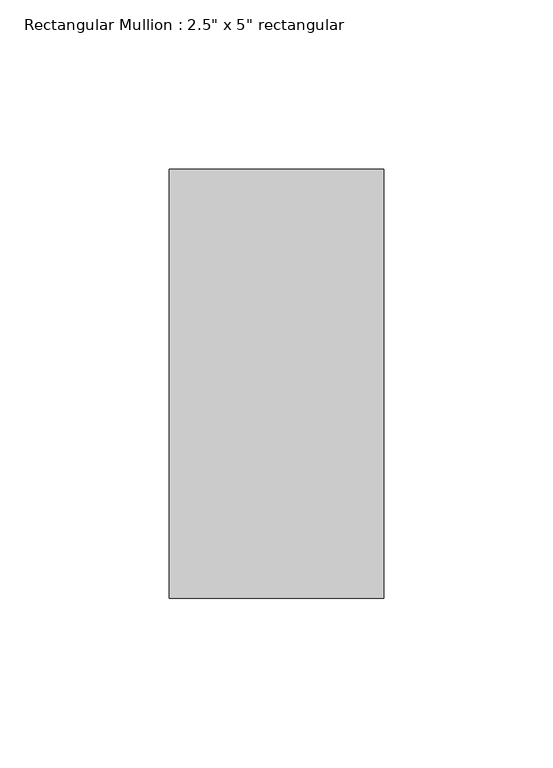
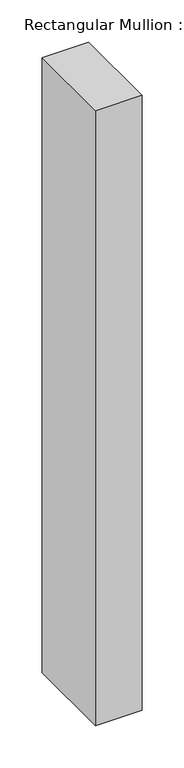
"""IFC4 building model written with IfcOpenShell, lengths in millimetres: member geometry."""

from ifc_helpers import new_model, si_unit, frame, origin, place, context, project, spatial, polyline, outline, extrude, source, transform, mapped, element, save


def member_6e431393(model_context):
    return source(origin(), model_context, "Body", "SweptSolid", [
        extrude(outline(polyline([(31.75, 63.5), (31.75, -63.5), (-31.75, -63.5), (-31.75, 63.5), (31.75, 63.5)])), frame((0.0, 0.0, -889.0), z_axis=(0.0, 0.0, 1.0), x_axis=(1.0, 0.0, 0.0)), (0.0, 0.0, 1.0), 889.0),
    ])


if __name__ == "__main__":
    model = new_model("IFC4")
    model_context = context("Model", 3, world=origin())
    ifc_project = project(units=[si_unit("LENGTHUNIT", "METRE", prefix="MILLI")], contexts=[model_context])
    site = spatial("IfcSite", under=ifc_project)
    building = spatial("IfcBuilding", under=site)
    placement = place(None, origin())
    member_shape = member_6e431393(model_context)
    element("IfcMember", 1, ObjectType="Rectangular Mullion : 2.5\" x 5\" rectangular", at=placement, inside=building, context=model_context, shape_type="MappedRepresentation", body=[
        mapped(member_shape, transform((0.0, 0.0, 0.0), x_axis=(1.0, 0.0, 0.0), y_axis=(0.0, 1.0, 0.0), z_axis=(0.0, 0.0, 1.0))),
    ])
    save(model, "model.ifc")

# Revit data of these elements
# Type "Rectangular Mullion : 2.5\" x 5\" rectangular"
#   built-in parameter 1007304 = 0.416667 (stored number, unit not read)
#   built-in parameter 1007301 = 0.104167 (stored number, unit not read)
#   built-in parameter 1007300 = 0.104167 (stored number, unit not read)
# Element 1 (IfcMember, "Rectangular Mullion : 2.5\" x 5\" rectangular")
#   Materials on its faces: "Aluminum"
# Materials
#   "Aluminum": class "Metal", colour RGB 247 247 247, transparency 0, Description = "Aluminum 6061", Cost = 0
